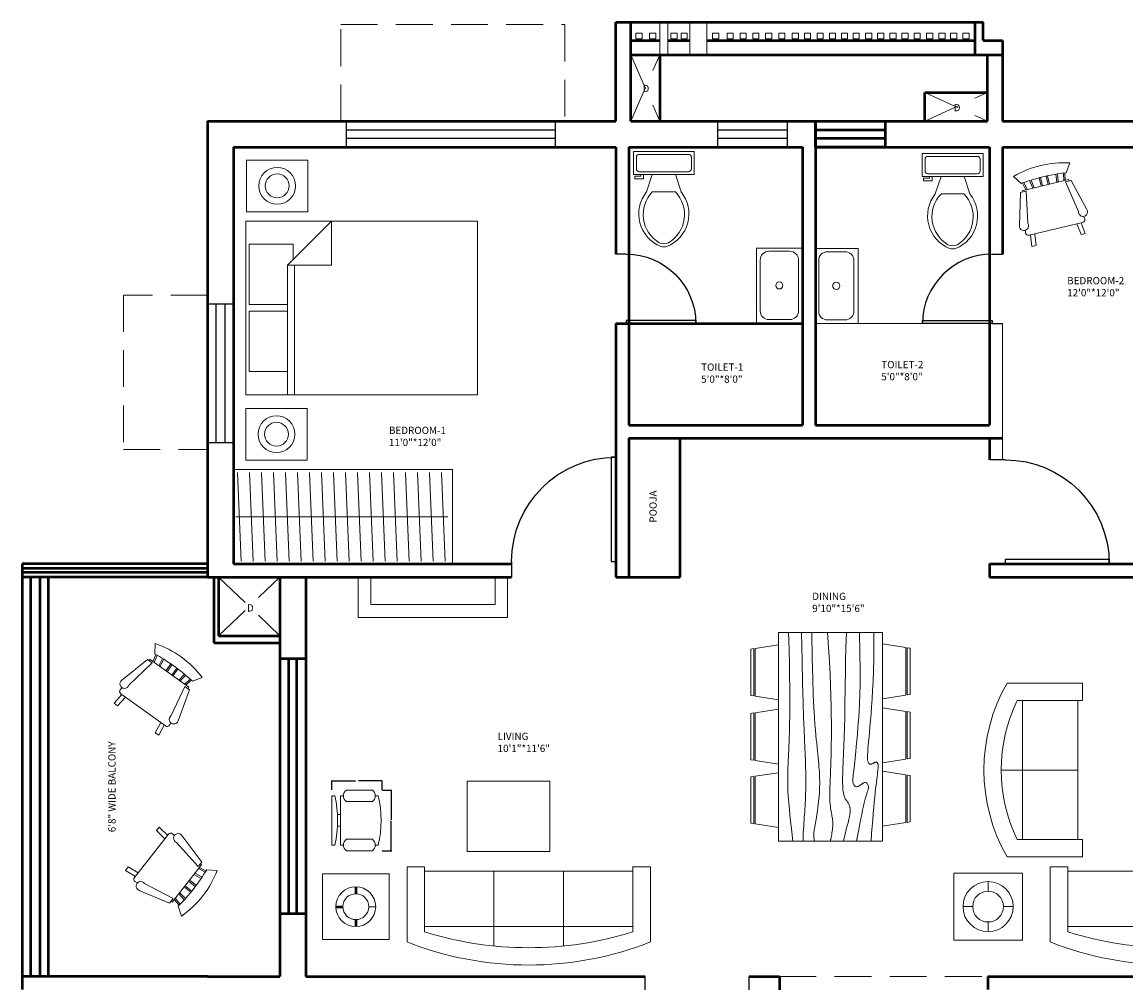
# Model space of a CAD drawing. Units: inches. Extents: x 4795 to 6024, y 2716 to 5025.
# Tile 13 of 19: x 4795 to 5177, y 4676 to 5008. Entities that reach past the tile are written whole.
import ezdxf

# ---------------------------------------------------------------- set-up
doc = ezdxf.new("R2010")
doc.units = ezdxf.units.IN
doc.linetypes.add('DASHED', pattern=[19.05, 12.7, -6.35])
for name, color, linetype, lineweight in [('A-ANNO-DIMS', 2, 'Continuous', 18), ('A-ANNO-TEXT', 7, 'Continuous', 18), ('A-AREA-IDEN', 3, 'Continuous', 18), ('A-DOOR', 4, 'Continuous', 25), ('A-FLOR-FIXT', 9, 'Continuous', 18), ('A-FURN', 8, 'Continuous', 18), ('A-GLAZ', 4, 'Continuous', 25), ('A-WALL', 7, 'Continuous', 50), ('A-WALL-OVHD', 8, 'DASHED', 18)]:
    doc.layers.add(name, color=color, linetype=linetype, lineweight=lineweight)
doc.styles.get("Standard").update_dxf_attribs({"font": 'arial.ttf'})
doc.dimstyles.get("Standard").update_dxf_attribs({"dimtxt": 0.18, "dimasz": 0.18, "dimexe": 0.18, "dimexo": 0.0625, "dimgap": 0.09, "dimtad": 0, "dimtih": 1, "dimtoh": 1, "dimdec": 4, "dimzin": 0, "dimdsep": 46, "dimtxsty": 'Standard', "dimcen": 0.09, "dimadec": 0, "dimazin": 0, "dimtfac": 1, "dimtdec": 4, "dimtofl": 0, "dimtmove": 0, "dimatfit": 3, "dimfxl": 1, "dimtolj": 1, "dimtzin": 0, "dimarcsym": 0})

# ---------------------------------------------------------------- blocks, each defined once
blk = doc.blocks.new('*U2')
for p, q in [((0, 0), (0, -6)), ((40, 0), (40, -6))]:
    blk.add_line(p, q)
blk.add_lwpolyline([(0, 0), (0, 40), (1.75, 40), (1.75, 0)], close=True)
blk.add_arc((0, 0), 40, 0, 90)
blk = doc.blocks.new('Bed - Queen')
for p, q in [((0, -80.00003), (0, 0)), ((0, 0), (59.99999, 0)), ((59.99999, 0), (59.99999, -80.00003)), ((7.99999, -1.2), (28.79998, -1.2)), ((7.99999, -14.4), (7.99999, -1.2)), ((28.79998, -1.2), (28.79998, -14.4)), ((31.19999, -1.2), (51.99999, -1.2)), ((31.19999, -14.4), (31.19999, -1.2)), ((51.99999, -1.2), (51.99999, -16.4)), ((0, -14.4), (44.8, -14.4)), ((59.99999, -29.6), (44.8, -14.4)), ((44.8, -14.4), (44.8, -29.6)), ((44.8, -16.8), (0, -16.8)), ((51.99999, -16.4), (46.79936, -16.4)), ((44.8, -29.6), (59.99999, -29.6)), ((59.99999, -80.00003), (0, -80.00003))]:
    blk.add_line(p, q)
blk = doc.blocks.new('Toilet - top')
for p, q in [((9.5, -6), (9.5, -2)), ((-10, -8.5), (-8, -8.5)), ((-10, -9.5), (-10, -8.5)), ((-7, -9.5), (-10, -9.5)), ((-8, -8.5), (-8, -8)), ((-7, -8), (-7, -9.5)), ((-4, -8), (-6, -14)), ((4, -8), (6, -14)), ((4, -14), (-4, -14))]:
    blk.add_line(p, q)
blk.add_lwpolyline([(10.5, -8), (10.5, 0), (-10.5, 0), (-10.5, -8)], close=True)
for points in [[(-9.5, -2), (-9.5, -6)], [(8.5, -1), (-8.5, -1)], [(-8.5, -7), (8.5, -7)]]:
    blk.add_lwpolyline(points)
for centre, radius, start, end in [((-8.62, -1.88), 0.884, 81.8699, 188.1301), ((8.62, -1.88), 0.884, 351.8699, 98.1301), ((-8.62, -6.12), 0.884, 171.8699, 278.1301), ((8.62, -6.12), 0.884, 261.8699, 8.1301), ((3.52, -21.58), 12.17, 141.4691, 247.9714), ((4.2, -21.82), 11.33, 136.3677, 238.9468), ((-3.52, -21.58), 12.17, 292.0284, 38.5307), ((-4.2, -21.82), 11.33, 301.053, 43.6321), ((0, -27.88), 4, 245.7318, 294.2682), ((0, -29), 4, 254.8605, 285.1395)]:
    blk.add_arc(centre, radius, start, end)
blk = doc.blocks.new('Sofa - Roundback 7 ft.')
for p, q in [((-12.00002, -32.4421), (-12.00003, -6.5971)), ((11.99997, -32.4421), (11.99998, -6.5971)), ((-36.000027, -34), (-36.000027, -11.4696)), ((-35.999844, -13.3819), (35.9998, -13.3819)), ((35.99998, -34), (35.99998, -11.4696)), ((-36.000027, -32.4421), (35.99998, -32.4421))]:
    blk.add_line(p, q)
for points in [[(-36.000027, -34), (-42.000027, -34), (-42.000027, -8)], [(41.99998, -8), (41.99998, -34), (35.99998, -34)]]:
    blk.add_lwpolyline(points)
for centre, radius, start, end in [((0, -114.25), 114.25, 68.43141, 111.5686), ((-0.00001, -127.1968), 121.1968, 72.72033, 107.2797)]:
    blk.add_arc(centre, radius, start, end)
blk = doc.blocks.new('Chair - Desk')
for p, q in [((-8.5, 0), (-8.5, -1)), ((-8.5, 0), (8.5, 0)), ((8.5, 0), (8.5, -1)), ((-8.5, -3), (-8.5, -4)), ((-8.5, -3), (8.5, -3)), ((-2, -3), (-2, -1.9355)), ((2, -1.9576), (2, -3)), ((8.5, -3), (8.5, -4)), ((-10.5, -5), (-10.5, -14)), ((-6.5, -14), (-6.5, -5)), ((6.5, -5), (6.5, -14)), ((10.5, -14), (10.5, -5)), ((-8.5, -15), (-8.5, -16)), ((8.5, -15), (8.5, -16))]:
    blk.add_line(p, q)
for centre, radius, start, end in [((0, 34.625), 36.625, 256.5803, 283.4197), ((-8.5, -6.5), 2.5, 36.8699, 143.1301), ((8.5, -6.5), 2.5, 36.8699, 143.1301), ((-8.5, -12.5), 2.5, 216.8699, 323.1301), ((8.5, -12.5), 2.5, 216.8699, 323.1301), ((0, 19.625), 36.625, 256.5803, 283.4197)]:
    blk.add_arc(centre, radius, start, end)
blk = doc.blocks.new('Sofa - Roundback Loveseat 5 ft.')
for p, q in [((0, -32.44198), (0, -5.99998)), ((-24, -33.99998), (-24, -11.46958)), ((-23.9998, -13.38178), (23.99986, -13.38178)), ((24.00004, -33.99998), (24.00004, -11.46958)), ((-24, -32.44198), (24.00004, -32.44198))]:
    blk.add_line(p, q)
for points in [[(-24, -33.99998), (-30, -33.99998), (-30, -7.99998)], [(30.00004, -7.99998), (30.00004, -33.99998), (24.00004, -33.99998)]]:
    blk.add_lwpolyline(points)
for centre, radius, start, end in [((0, -60.24998), 60.24998, 60.13715, 119.8628), ((0, -61.38438), 55.38444, 64.32083, 115.6792)]:
    blk.add_arc(centre, radius, start, end)
blk = doc.blocks.new('Chair - Rocking')
for p, q in [((-8, -4.5), (-10, -1.5)), ((8, -4.5), (10, -1.5)), ((-9, -7.5), (-12, -18.49999)), ((-7, -7.5), (-9, -7.5)), ((-9, -18.49999), (-7, -7.5)), ((-8.23428, -6.99939), (-8.3093, -7.47958)), ((-8.23041, -7), (8.23915, -7)), ((-7.5, -4.5), (-7, -7)), ((-6.5, -7), (-7.02225, -4.43)), ((-4.5, -7), (-4.96674, -4.19951)), ((-4, -7), (-4.40532, -4.16272)), ((-1.5, -4.05012), (-1.5, -7)), ((-1, -7), (-1, -4.05012)), ((1, -7), (1, -4.04655)), ((1.5, -4.05012), (1.5, -7)), ((4, -7), (4.40187, -4.18694)), ((4.5, -7), (4.96761, -4.19437)), ((6.5, -7), (7, -4.4057)), ((7.5, -4.5), (7, -7)), ((7, -7.5), (9, -7.5)), ((9, -18.49999), (7, -7.5)), ((8.31071, -7.48854), (8.23449, -7.00073)), ((9, -7.5), (12, -18.49999)), ((-10.36644, -20.64523), (-10.5, -21.49999)), ((-9, -22.49999), (-9.5, -26.49999)), ((0, -22.49999), (-9.5, -22.49999)), ((-8, -26.49999), (-7.5, -22.49999)), ((0, -22.49999), (9.5, -22.49999)), ((8, -26.49999), (7.5, -22.49999)), ((9, -22.49999), (9.5, -26.49999)), ((10.5, -21.49999), (10.3575, -20.58798)), ((-9.5, -26.49999), (-8, -26.49999)), ((9.5, -26.49999), (8, -26.49999))]:
    blk.add_line(p, q)
for centre, radius, start, end in [((0, -34.08333), 34.08333, 72.93847, 107.0615), ((0, -68.25004), 64.25, 93.92211, 97.15267), ((0, -68.25004), 64.25, 82.84733, 93.92211), ((-10.5, -18.99999), 1.58114, 161.5651, 18.43495), ((10.5, -18.99999), 1.58114, 161.5651, 18.43495), ((-9.5, -21.49999), 1, 180, 270), ((9.5, -21.49999), 1, 270, 0)]:
    blk.add_arc(centre, radius, start, end)
blk = doc.blocks.new('WIN-48')
for p, q in [((0, 0), (0, 48)), ((0, 48), (9, 48)), ((3, 0), (3, 48)), ((6, 48), (6, 0)), ((9, 48), (9, 0)), ((9, 0), (0, 0))]:
    blk.add_line(p, q)
blk = doc.blocks.new('WIN-72')
for p, q in [((0, 0), (0, 9)), ((0, 9), (72, 9)), ((72, 9), (72, 0)), ((0, 6), (72, 6)), ((72, 3), (0, 3)), ((72, 0), (0, 0))]:
    blk.add_line(p, q)
blk = doc.blocks.new('WIN-24')
for p, q in [((0, 0), (0, 9)), ((0, 9), (24, 9)), ((24, 9), (24, 0)), ((0, 6), (24, 6)), ((24, 3), (0, 3)), ((24, 0), (0, 0))]:
    blk.add_line(p, q)
blk = doc.blocks.new('CHAIR-DINING')
for p, q in [((8, 17.72), (0, 18.97)), ((8, 17.71), (8, 1.25)), ((9.5, 17.48), (8.5, 17.64)), ((8.5, 1.33), (8.5, 17.64)), ((9.5, 17.48), (9.5, 1.48)), ((0, 0), (8, 1.25)), ((8.5, 1.33), (9.5, 1.48))]:
    blk.add_line(p, q)
blk = doc.blocks.new('LAMP-SIDE')
for p, q in [((11.88, 20.25), (11.88, 16.92)), ((3.23, 11.6), (6.56, 11.6)), ((17.2, 11.6), (20.54, 11.6)), ((11.88, 6.28), (11.88, 2.94))]:
    blk.add_line(p, q)
blk.add_lwpolyline([(23.76, 23.19), (0, 23.19), (0, 0), (23.76, 0)], close=True)
for radius in [8.66, 5.32]:
    blk.add_circle((11.88, 11.6), radius)
blk = doc.blocks.new('*D19')
at = {"layer": 'A-ANNO-DIMS', "color": 0, "lineweight": -2, "transparency": 16777216}
for p, q in [((4919.79, 4742.88), (4923.06, 4742.88)), ((4922.88, 4742.7), (4922.88, 4732.56)), ((4922.88, 4722.06), (4922.88, 4732.2)), ((4919.79, 4721.88), (4923.06, 4721.88))]:
    blk.add_line(p, q, dxfattribs=at)
at = {"layer": 'A-ANNO-DIMS', "color": 0, "lineweight": 100, "transparency": 16777216}
for points in [[(4922.85, 4742.7), (4922.91, 4742.7), (4922.88, 4742.88)], [(4922.85, 4722.06), (4922.91, 4722.06), (4922.88, 4721.88)]]:
    blk.add_solid(points, dxfattribs=at)
at = {"layer": 'DEFPOINTS', "color": 0, "lineweight": 100, "transparency": 16777216}
for p in [(4919.73, 4742.88), (4922.88, 4742.88), (4919.73, 4721.88)]:
    blk.add_point(p, dxfattribs=at)
at = {"layer": 'A-ANNO-DIMS', "color": 0, "transparency": 16777216, "insert": (4922.88, 4732.38), "char_height": 0.18, "attachment_point": 5}
blk.add_mtext('\\A1;DESK CHAIR 21 TYP.', dxfattribs=at)
blk = doc.blocks.new('*D20')
at = {"layer": 'A-ANNO-DIMS', "color": 0, "lineweight": -2, "transparency": 16777216}
for p, q in [((4902.4, 4742.94), (4902.4, 4746.21)), ((4902.58, 4746.03), (4910.54, 4746.03)), ((4919.55, 4746.03), (4911.58, 4746.03)), ((4919.73, 4742.94), (4919.73, 4746.21))]:
    blk.add_line(p, q, dxfattribs=at)
at = {"layer": 'A-ANNO-DIMS', "color": 0, "lineweight": 100, "transparency": 16777216}
for points in [[(4902.58, 4746.06), (4902.58, 4746), (4902.4, 4746.03)], [(4919.55, 4746.06), (4919.55, 4746), (4919.73, 4746.03)]]:
    blk.add_solid(points, dxfattribs=at)
at = {"layer": 'DEFPOINTS', "color": 0, "lineweight": 100, "transparency": 16777216}
for p in [(4902.4, 4746.03), (4902.4, 4742.88), (4919.73, 4742.88)]:
    blk.add_point(p, dxfattribs=at)
at = {"layer": 'A-ANNO-DIMS', "color": 0, "transparency": 16777216, "insert": (4911.06, 4746.03), "char_height": 0.18, "attachment_point": 5}
blk.add_mtext('\\A1;17 TYP.', dxfattribs=at)

msp = doc.modelspace()

# ---------------------------------------------------------------- linework, layer by layer
at = {"layer": 'A-FLOR-FIXT'}
for points in [[(5064.97, 4904.04), (5049.09, 4904.04), (5049.09, 4930.14), (5064.97, 4930.14)], [(5069.47, 4904.04), (5084.11, 4904.04), (5084.11, 4929.94), (5069.47, 4929.94)]]:
    msp.add_lwpolyline(points, close=True, dxfattribs=at)
for points in [[(5053.31, 4929.01), (5060.55, 4929.01, -0.414214), (5063.55, 4926.01), (5063.55, 4908.43, -0.414214), (5060.55, 4905.43), (5053.31, 4905.43, -0.414214), (5050.31, 4908.43), (5050.31, 4926.01, -0.414214)], [(5073.51, 4928.86), (5079.66, 4928.86, -0.414214), (5082.66, 4925.86), (5082.66, 4908.32, -0.414214), (5079.66, 4905.32), (5073.51, 4905.32, -0.414214), (5070.51, 4908.32), (5070.51, 4925.86, -0.414214)]]:
    msp.add_lwpolyline(points, format="xyb", close=True, dxfattribs=at)
for centre, radius in [((5056.93, 4917.22), 1.22), ((5076.59, 4917.09), 1.24)]:
    msp.add_circle(centre, radius, dxfattribs=at)
at = {"layer": 'A-FURN'}
for p, q in [((5069.47, 4904.04), (5133.97, 4904.04)), ((5133.97, 4904.04), (5133.97, 4856.98)), ((4868.47, 4853.67), (4944.05, 4853.67)), ((4869.87, 4852.58), (4871.08, 4821.91)), ((4874.01, 4852.58), (4875.23, 4821.91)), ((4878.15, 4852.58), (4879.37, 4821.91)), ((4882.3, 4852.58), (4883.51, 4821.91)), ((4886.44, 4852.58), (4887.66, 4821.91)), ((4890.58, 4852.58), (4891.8, 4821.91)), ((4894.73, 4852.58), (4895.94, 4821.91)), ((4898.87, 4852.58), (4900.09, 4821.91)), ((4903.02, 4852.58), (4904.23, 4821.91)), ((4907.16, 4852.58), (4908.38, 4821.91)), ((4911.3, 4852.58), (4912.52, 4821.91)), ((4915.45, 4852.58), (4916.66, 4821.91)), ((4919.59, 4852.58), (4920.81, 4821.91)), ((4923.73, 4852.58), (4924.95, 4821.91)), ((4927.88, 4852.58), (4929.09, 4821.91)), ((4932.02, 4852.58), (4933.24, 4821.91)), ((4936.17, 4852.58), (4937.38, 4821.91)), ((4940.31, 4852.58), (4941.53, 4821.91)), ((4944.05, 4853.67), (4944.05, 4820.98)), ((4869.24, 4837.25), (4942.48, 4837.25)), ((4911.47, 4816.48), (4911.47, 4802.48)), ((4915.82, 4816.48), (4915.82, 4806.99)), ((4958.77, 4806.99), (4958.77, 4816.48)), ((4963.08, 4802.48), (4963.08, 4816.48)), ((4915.82, 4806.99), (4958.77, 4806.99)), ((4911.47, 4802.48), (4963.08, 4802.48)), ((5056.6, 4797.26), (5056.6, 4725.26)), ((5092.6, 4797.26), (5056.6, 4797.26)), ((5092.6, 4725.26), (5092.6, 4797.26)), ((5056.6, 4725.26), (5092.6, 4725.26)), ((4915.14, 4702.58), (4917.55, 4702.58))]:
    msp.add_line(p, q, dxfattribs=at)
for points in [[(5015.65, 5008.22), (5018.42, 5008.22), (5018.42, 4996.94), (5015.65, 4996.94)], [(5026.04, 5008.22), (5031.9, 5008.22), (5031.9, 4996.94), (5026.04, 4996.94)], [(5007.39, 5004.38), (5009.52, 5004.38), (5009.52, 5002.46), (5007.39, 5002.46)], [(5012.14, 5004.38), (5014.27, 5004.38), (5014.27, 5002.46), (5012.14, 5002.46)], [(5019.47, 5004.38), (5021.6, 5004.38), (5021.6, 5002.46), (5019.47, 5002.46)], [(5022.98, 5004.38), (5025.1, 5004.38), (5025.1, 5002.46), (5022.98, 5002.46)], [(5033.88, 5004.38), (5036, 5004.38), (5036, 5002.46), (5033.88, 5002.46)], [(5038.86, 5004.38), (5040.99, 5004.38), (5040.99, 5002.46), (5038.86, 5002.46)], [(5043.35, 5004.38), (5045.47, 5004.38), (5045.47, 5002.46), (5043.35, 5002.46)], [(5047.73, 5004.38), (5049.86, 5004.38), (5049.86, 5002.46), (5047.73, 5002.46)], [(5052.19, 5004.38), (5054.32, 5004.38), (5054.32, 5002.46), (5052.19, 5002.46)], [(5056.71, 5004.38), (5058.83, 5004.38), (5058.83, 5002.46), (5056.71, 5002.46)], [(5061.36, 5004.38), (5063.49, 5004.38), (5063.49, 5002.46), (5061.36, 5002.46)], [(5065.58, 5004.38), (5067.71, 5004.38), (5067.71, 5002.46), (5065.58, 5002.46)], [(5069.98, 5004.38), (5072.1, 5004.38), (5072.1, 5002.46), (5069.98, 5002.46)], [(5074.23, 5004.38), (5076.36, 5004.38), (5076.36, 5002.46), (5074.23, 5002.46)], [(5078.38, 5004.38), (5080.51, 5004.38), (5080.51, 5002.46), (5078.38, 5002.46)], [(5082.37, 5004.38), (5084.5, 5004.38), (5084.5, 5002.46), (5082.37, 5002.46)], [(5086.69, 5004.38), (5088.82, 5004.38), (5088.82, 5002.46), (5086.69, 5002.46)], [(5090.88, 5004.38), (5093.01, 5004.38), (5093.01, 5002.46), (5090.88, 5002.46)], [(5095.1, 5004.38), (5097.23, 5004.38), (5097.23, 5002.46), (5095.1, 5002.46)], [(5099.26, 5004.38), (5101.38, 5004.38), (5101.38, 5002.46), (5099.26, 5002.46)], [(5103.48, 5004.38), (5105.61, 5004.38), (5105.61, 5002.46), (5103.48, 5002.46)], [(5107.77, 5004.38), (5109.9, 5004.38), (5109.9, 5002.46), (5107.77, 5002.46)], [(5112.06, 5004.38), (5114.18, 5004.38), (5114.18, 5002.46), (5112.06, 5002.46)], [(5116.08, 5004.38), (5118.2, 5004.38), (5118.2, 5002.46), (5116.08, 5002.46)], [(5120.33, 5004.38), (5122.46, 5004.38), (5122.46, 5002.46), (5120.33, 5002.46)], [(4872.88, 4960.54), (4894.15, 4960.54), (4894.15, 4942.71), (4872.88, 4942.71)], [(4872.65, 4874.74), (4893.91, 4874.74), (4893.91, 4856.91), (4872.65, 4856.91)], [(4949.08, 4745.98), (4977.63, 4745.98), (4977.63, 4721.64), (4949.08, 4721.64)], [(4899.19, 4713.94), (4922.15, 4713.94), (4922.15, 4691.23), (4899.19, 4691.23)]]:
    msp.add_lwpolyline(points, close=True, dxfattribs=at)
for points in [[(5060.1, 4797.26), (5060.27, 4791.35), (5060.39, 4786.3), (5060.48, 4781.99), (5060.53, 4778.34), (5060.56, 4775.23), (5060.56, 4772.57), (5060.55, 4770.24), (5060.52, 4768.14), (5060.49, 4766.19), (5060.44, 4764.35), (5060.4, 4762.63), (5060.34, 4761.02), (5060.29, 4759.5), (5060.23, 4758.07), (5060.17, 4756.71), (5060.1, 4755.43), (5060.04, 4754.21), (5059.98, 4753.03), (5059.93, 4751.87), (5059.88, 4750.72), (5059.84, 4749.54), (5059.82, 4748.33), (5059.81, 4747.07), (5059.81, 4745.72), (5059.84, 4744.27), (5059.9, 4742.65), (5060, 4740.78), (5060.16, 4738.6), (5060.39, 4736.03), (5060.7, 4733), (5061.1, 4729.44), (5061.6, 4725.26)], [(5064.6, 4797.26), (5064.79, 4787.67), (5064.98, 4779.73), (5065.15, 4773.25), (5065.32, 4768), (5065.48, 4763.79), (5065.62, 4760.38), (5065.75, 4757.59), (5065.85, 4755.18), (5065.94, 4752.99), (5066, 4750.96), (5066.04, 4749.09), (5066.06, 4747.37), (5066.07, 4745.78), (5066.06, 4744.3), (5066.05, 4742.94), (5066.02, 4741.68), (5065.99, 4740.5), (5065.94, 4739.39), (5065.89, 4738.34), (5065.84, 4737.34), (5065.78, 4736.35), (5065.71, 4735.39), (5065.64, 4734.42), (5065.56, 4733.43), (5065.48, 4732.42), (5065.4, 4731.38), (5065.33, 4730.33), (5065.26, 4729.28), (5065.19, 4728.24), (5065.15, 4727.22), (5065.12, 4726.22), (5065.1, 4725.26)], [(5068.1, 4797.26), (5068.29, 4788.45), (5068.48, 4781.35), (5068.66, 4775.73), (5068.84, 4771.37), (5069.02, 4768.04), (5069.19, 4765.5), (5069.36, 4763.53), (5069.52, 4761.89), (5069.67, 4760.39), (5069.82, 4758.99), (5069.95, 4757.68), (5070.08, 4756.43), (5070.2, 4755.26), (5070.32, 4754.14), (5070.42, 4753.06), (5070.52, 4752.01), (5070.61, 4750.99), (5070.69, 4749.99), (5070.76, 4749), (5070.81, 4748.01), (5070.85, 4747.03), (5070.87, 4746.04), (5070.87, 4745.03), (5070.85, 4744.01), (5070.81, 4742.97), (5070.75, 4741.92), (5070.67, 4740.86), (5070.57, 4739.82), (5070.47, 4738.79), (5070.35, 4737.79), (5070.23, 4736.83), (5070.1, 4735.93), (5069.98, 4735.08), (5069.85, 4734.29), (5069.73, 4733.55), (5069.61, 4732.84), (5069.49, 4732.16), (5069.37, 4731.51), (5069.26, 4730.86), (5069.15, 4730.22), (5069.04, 4729.58), (5068.95, 4728.94), (5068.87, 4728.3), (5068.83, 4727.66), (5068.82, 4727.04), (5068.86, 4726.43), (5068.95, 4725.84), (5069.1, 4725.26)], [(5073.6, 4797.26), (5073.94, 4792.05), (5074.22, 4787.28), (5074.44, 4782.91), (5074.61, 4778.92), (5074.73, 4775.26), (5074.82, 4771.92), (5074.87, 4768.84), (5074.9, 4766.01), (5074.9, 4763.4), (5074.89, 4760.98), (5074.87, 4758.73), (5074.83, 4756.65), (5074.78, 4754.71), (5074.73, 4752.9), (5074.67, 4751.2), (5074.6, 4749.6), (5074.54, 4748.07), (5074.48, 4746.63), (5074.43, 4745.26), (5074.39, 4743.98), (5074.35, 4742.78), (5074.33, 4741.66), (5074.33, 4740.63), (5074.35, 4739.68), (5074.4, 4738.81), (5074.46, 4738.03), (5074.54, 4737.31), (5074.62, 4736.65), (5074.72, 4736.04), (5074.82, 4735.47), (5074.92, 4734.94), (5075.02, 4734.43), (5075.11, 4733.94), (5075.19, 4733.45), (5075.26, 4732.97), (5075.31, 4732.49), (5075.35, 4732), (5075.37, 4731.5), (5075.37, 4730.98), (5075.35, 4730.43), (5075.31, 4729.85), (5075.25, 4729.26), (5075.18, 4728.67), (5075.09, 4728.1), (5075.01, 4727.56), (5074.92, 4727.07), (5074.84, 4726.65), (5074.77, 4726.3), (5074.72, 4726.05), (5074.67, 4725.88), (5074.64, 4725.76), (5074.62, 4725.67), (5074.61, 4725.6), (5074.61, 4725.53), (5074.6, 4725.42), (5074.6, 4725.26)], [(5080.1, 4797.26), (5079.94, 4791.98), (5079.81, 4787.33), (5079.72, 4783.26), (5079.66, 4779.69), (5079.61, 4776.56), (5079.58, 4773.81), (5079.55, 4771.37), (5079.52, 4769.18), (5079.49, 4767.17), (5079.44, 4765.32), (5079.4, 4763.61), (5079.34, 4762), (5079.29, 4760.49), (5079.23, 4759.04), (5079.17, 4757.64), (5079.1, 4756.26), (5079.04, 4754.89), (5078.98, 4753.53), (5078.93, 4752.19), (5078.87, 4750.89), (5078.83, 4749.63), (5078.8, 4748.43), (5078.78, 4747.31), (5078.77, 4746.26), (5078.78, 4745.31), (5078.8, 4744.44), (5078.84, 4743.66), (5078.9, 4742.96), (5078.97, 4742.33), (5079.05, 4741.77), (5079.15, 4741.28), (5079.27, 4740.85), (5079.4, 4740.47), (5079.55, 4740.13), (5079.7, 4739.84), (5079.86, 4739.58), (5080.03, 4739.34), (5080.2, 4739.11), (5080.36, 4738.9), (5080.52, 4738.68), (5080.67, 4738.46), (5080.81, 4738.22), (5080.95, 4737.98), (5081.06, 4737.71), (5081.16, 4737.43), (5081.25, 4737.12), (5081.31, 4736.79), (5081.35, 4736.43), (5081.37, 4736.04), (5081.37, 4735.62), (5081.35, 4735.18), (5081.3, 4734.71), (5081.24, 4734.23), (5081.15, 4733.72), (5081.05, 4733.21), (5080.94, 4732.68), (5080.8, 4732.14), (5080.65, 4731.56), (5080.47, 4730.9), (5080.27, 4730.13), (5080.04, 4729.21), (5079.77, 4728.12), (5079.46, 4726.82), (5079.1, 4725.26)], [(5084.6, 4797.26), (5084.75, 4790.24), (5084.81, 4784.44), (5084.8, 4779.69), (5084.74, 4775.83), (5084.63, 4772.7), (5084.5, 4770.14), (5084.35, 4767.98), (5084.19, 4766.05), (5084.03, 4764.23), (5083.89, 4762.49), (5083.75, 4760.82), (5083.61, 4759.24), (5083.48, 4757.74), (5083.36, 4756.32), (5083.23, 4755), (5083.1, 4753.76), (5082.98, 4752.62), (5082.86, 4751.57), (5082.74, 4750.61), (5082.64, 4749.73), (5082.54, 4748.94), (5082.46, 4748.22), (5082.4, 4747.58), (5082.35, 4747.01), (5082.33, 4746.52), (5082.34, 4746.08), (5082.36, 4745.71), (5082.41, 4745.39), (5082.47, 4745.11), (5082.55, 4744.88), (5082.65, 4744.68), (5082.77, 4744.51), (5082.9, 4744.37), (5083.05, 4744.25), (5083.21, 4744.15), (5083.37, 4744.09), (5083.55, 4744.04), (5083.73, 4744.03), (5083.92, 4744.05), (5084.1, 4744.1), (5084.29, 4744.17), (5084.48, 4744.28), (5084.67, 4744.4), (5084.85, 4744.53), (5085.04, 4744.68), (5085.23, 4744.82), (5085.42, 4744.96), (5085.6, 4745.1), (5085.79, 4745.21), (5085.98, 4745.31), (5086.16, 4745.39), (5086.34, 4745.44), (5086.52, 4745.46), (5086.69, 4745.46), (5086.86, 4745.42), (5087.02, 4745.35), (5087.17, 4745.23), (5087.31, 4745.08), (5087.44, 4744.9), (5087.54, 4744.69), (5087.62, 4744.45), (5087.68, 4744.19), (5087.7, 4743.9), (5087.69, 4743.6), (5087.64, 4743.27), (5087.55, 4742.92), (5087.43, 4742.52), (5087.29, 4742.07), (5087.11, 4741.54), (5086.92, 4740.93), (5086.71, 4740.22), (5086.48, 4739.39), (5086.24, 4738.43), (5085.98, 4737.3), (5085.69, 4735.98), (5085.37, 4734.43), (5085.01, 4732.62), (5084.6, 4730.51), (5084.13, 4728.07), (5083.6, 4725.26)], [(5089.6, 4797.26), (5089.58, 4792.44), (5089.52, 4788.07), (5089.42, 4784.12), (5089.29, 4780.54), (5089.14, 4777.3), (5088.97, 4774.36), (5088.79, 4771.68), (5088.6, 4769.22), (5088.42, 4766.95), (5088.23, 4764.87), (5088.06, 4762.96), (5087.9, 4761.23), (5087.75, 4759.67), (5087.62, 4758.28), (5087.51, 4757.06), (5087.44, 4756.01), (5087.39, 4755.12), (5087.37, 4754.38), (5087.38, 4753.77), (5087.42, 4753.28), (5087.47, 4752.89), (5087.55, 4752.59), (5087.65, 4752.36), (5087.77, 4752.18), (5087.9, 4752.04), (5088.05, 4751.94), (5088.2, 4751.87), (5088.36, 4751.84), (5088.53, 4751.83), (5088.7, 4751.84), (5088.86, 4751.88), (5089.02, 4751.93), (5089.17, 4752), (5089.32, 4752.08), (5089.46, 4752.17), (5089.59, 4752.25), (5089.72, 4752.34), (5089.85, 4752.41), (5089.98, 4752.47), (5090.1, 4752.51), (5090.23, 4752.53), (5090.35, 4752.53), (5090.47, 4752.5), (5090.58, 4752.45), (5090.69, 4752.38), (5090.78, 4752.28), (5090.87, 4752.16), (5090.94, 4752.01), (5090.99, 4751.84), (5091.03, 4751.65), (5091.05, 4751.41), (5091.06, 4751.14), (5091.05, 4750.82), (5091.03, 4750.44), (5090.99, 4750.01), (5090.94, 4749.51), (5090.87, 4748.94), (5090.78, 4748.29), (5090.68, 4747.55), (5090.57, 4746.7), (5090.45, 4745.72), (5090.32, 4744.62), (5090.17, 4743.37), (5090.02, 4741.97), (5089.86, 4740.4), (5089.69, 4738.68), (5089.52, 4736.79), (5089.34, 4734.76), (5089.16, 4732.58), (5088.98, 4730.27), (5088.79, 4727.83), (5088.6, 4725.26)]]:
    msp.add_lwpolyline(points, dxfattribs=at)
for centre, radius in [((4883.52, 4951.63), 6.37), ((4883.52, 4951.63), 4.11), ((4883.28, 4865.82), 6.37), ((4883.28, 4865.82), 4.11), ((4910.67, 4702.58), 6.88), ((4910.67, 4702.58), 4.47)]:
    msp.add_circle(centre, radius, dxfattribs=at)
at = {"layer": 'A-WALL'}
for p, q in [((5000.47, 4973.98), (5000.47, 5008.22)), ((5000.47, 5008.22), (5127.34, 5008.22)), ((5005.65, 4973.98), (5005.65, 5008.22)), ((5124.46, 5008.22), (5124.46, 4996.94)), ((5127.34, 5001.88), (5127.34, 5008.22)), ((5005.65, 5001.88), (5015.65, 5001.88)), ((5018.42, 5001.88), (5026.04, 5001.88)), ((5031.9, 5001.88), (5124.46, 5001.88)), ((5127.34, 5001.88), (5133.97, 5001.88)), ((5133.97, 5001.88), (5133.97, 4973.98)), ((5005.65, 4996.94), (5133.97, 4996.94)), ((5015.65, 4996.94), (5015.65, 4973.98)), ((5128.82, 4973.98), (5128.82, 4996.94)), ((5107.16, 4973.98), (5107.16, 4983.85)), ((5107.16, 4983.85), (5128.82, 4983.85)), ((4859.47, 4973.98), (4859.47, 4816.48)), ((4859.47, 4973.98), (5000.47, 4973.98)), ((5005.65, 4973.98), (5128.82, 4973.98)), ((5069.47, 4973.98), (5069.47, 4868.98)), ((5069.47, 4973.98), (5093.47, 4973.98)), ((5069.47, 4964.98), (5069.47, 4973.98)), ((5069.47, 4970.98), (5093.47, 4970.98)), ((5093.47, 4973.98), (5093.47, 4964.98)), ((5133.97, 4973.98), (5286.97, 4973.98)), ((5093.47, 4967.98), (5069.47, 4967.98)), ((4868.47, 4964.98), (5000.47, 4964.98)), ((4868.47, 4964.98), (4868.47, 4820.98)), ((5000.47, 4964.98), (5000.47, 4928.04)), ((5004.97, 4964.98), (5004.97, 4868.98)), ((5004.97, 4964.98), (5064.97, 4964.98)), ((5064.97, 4964.98), (5064.97, 4868.98)), ((5093.47, 4964.98), (5069.47, 4964.98)), ((5069.47, 4964.98), (5129.47, 4964.98)), ((5129.47, 4964.98), (5129.47, 4868.98)), ((5133.97, 4964.98), (5133.97, 4928.04)), ((5133.97, 4964.98), (5277.97, 4964.98)), ((5000.47, 4904.04), (5064.97, 4904.04)), ((5000.47, 4904.04), (5000.47, 4816.48)), ((5004.97, 4868.98), (5064.97, 4868.98)), ((5069.47, 4868.98), (5129.47, 4868.98)), ((5004.97, 4864.48), (5133.97, 4864.48)), ((5004.97, 4864.48), (5004.97, 4816.48)), ((5022.69, 4816.48), (5022.69, 4864.48)), ((5129.47, 4864.48), (5129.47, 4856.98)), ((4795.42, 4820.98), (4795.42, 4673.98)), ((4859.47, 4820.98), (4795.42, 4820.98)), ((4795.42, 4819.56), (4859.47, 4819.56)), ((4868.47, 4820.98), (4964.47, 4820.98)), ((5129.47, 4820.98), (5277.97, 4820.98)), ((5129.47, 4820.98), (5129.47, 4816.48)), ((4795.42, 4818.19), (4859.47, 4818.19)), ((4859.47, 4816.48), (4795.42, 4816.48)), ((4798.38, 4816.48), (4798.38, 4678.48)), ((4801.51, 4816.48), (4801.51, 4678.48)), ((4804.42, 4816.48), (4804.42, 4678.48)), ((4859.47, 4816.48), (4964.47, 4816.48)), ((4861.65, 4816.48), (4861.65, 4793.7)), ((4863.28, 4816.48), (4863.28, 4796.16)), ((4884.42, 4816.48), (4884.42, 4678.48)), ((4893.42, 4816.48), (4893.42, 4678.48)), ((5000.47, 4816.48), (5004.97, 4816.48)), ((5004.97, 4816.48), (5022.69, 4816.48)), ((5129.47, 4816.48), (5277.97, 4816.48)), ((4863.28, 4796.16), (4884.42, 4796.16)), ((4861.65, 4793.7), (4884.42, 4793.7)), ((4884.42, 4788.28), (4893.42, 4788.28)), ((4887.38, 4788.28), (4887.38, 4700.21)), ((4890.17, 4788.28), (4890.17, 4700.21)), ((4910.67, 4709.46), (4910.67, 4707.05)), ((4884.42, 4700.21), (4893.42, 4700.21)), ((4903.8, 4702.58), (4906.21, 4702.58)), ((4910.67, 4698.12), (4910.67, 4695.71)), ((4804.42, 4678.48), (4795.42, 4678.48)), ((4859.47, 4678.48), (4804.42, 4678.48)), ((4859.47, 4678.48), (4884.42, 4678.48)), ((4893.42, 4678.48), (5010.54, 4678.48)), ((5046.54, 4678.48), (5056.97, 4678.48)), ((5056.97, 4678.48), (5056.97, 4623.48)), ((5128.97, 4678.48), (5128.97, 4673.98)), ((5128.97, 4678.48), (5277.97, 4678.48))]:
    msp.add_line(p, q, dxfattribs=at)
at = {"layer": 'A-WALL-OVHD'}
for p, q in [((4905.5, 4973.98), (4905.5, 5007.33)), ((4905.5, 5007.33), (4982.88, 5007.33)), ((4982.88, 5007.33), (4982.88, 4973.98)), ((5005.65, 4996.94), (5015.65, 4973.98)), ((5005.65, 4973.98), (5015.65, 4996.94)), ((5107.16, 4983.85), (5128.82, 4973.98)), ((5107.16, 4973.98), (5128.82, 4983.85)), ((4859.47, 4913.89), (4830.42, 4913.89)), ((4830.42, 4913.89), (4830.42, 4860.52)), ((4830.42, 4860.52), (4859.47, 4860.52)), ((4863.28, 4816.48), (4884.42, 4796.16)), ((4863.28, 4796.16), (4884.42, 4816.48)), ((5056.97, 4678.48), (5128.97, 4678.48))]:
    msp.add_line(p, q, dxfattribs=at)

# ---------------------------------------------------------------- block references
at = {"layer": 'A-DOOR'}
for p, xscale, yscale, zscale, rotation in [((5004.07, 4904.04), -0.6, 0.6, 0.6, 270), ((5130.37, 4904.04), 0.6, 0.6, 0.6, 90.00000000000003), ((5134.87, 4820.98), -0.9, 0.9, 0.9, 270), ((5046.54, 4673.08), 0.9, 0.9, 0.9, 180)]:
    msp.add_blockref('*U2', p, dxfattribs=dict(at, xscale=xscale, yscale=yscale, zscale=zscale, rotation=rotation))
at = {"layer": 'A-DOOR', "xscale": -0.9, "yscale": 0.9, "zscale": 0.9}
msp.add_blockref('*U2', (5000.47, 4821.88), dxfattribs=at)
at = {"layer": 'A-FLOR-FIXT'}
for p in [(5017.05, 4963.52), (5116.76, 4962.82)]:
    msp.add_blockref('Toilet - top', p, dxfattribs=at)
at = {"layer": 'A-FURN'}
for name, p, rotation in [('Chair - Rocking', (5147.18, 4958.68), 13.47603948756063), ('Bed - Queen', (4872.65, 4879.48), 90), ('Chair - Rocking', (4850.37, 4788.86), 324.2775344515209), ('CHAIR-DINING', (5056.61, 4793.06), 180.0056718243519), ('Sofa - Roundback Loveseat 5 ft.', (5127.57, 4749.79), 90), ('CHAIR-DINING', (5056.61, 4770.84), 180.0056718243519), ('CHAIR-DINING', (5056.61, 4748.87), 180.0056718243519), ('Chair - Desk', (4902.4, 4732.38), 90), ('Chair - Rocking', (4857.82, 4706.29), 232.0049313276433), ('Sofa - Roundback 7 ft.', (4970.39, 4682.4), 180), ('Sofa - Roundback 7 ft.', (5192.5, 4682.4), 180)]:
    msp.add_blockref(name, p, dxfattribs=dict(at, rotation=rotation))
for name, p in [('CHAIR-DINING', (5092.6, 4774.43)), ('CHAIR-DINING', (5092.6, 4752.33)), ('CHAIR-DINING', (5092.6, 4730.39)), ('LAMP-SIDE', (5117.14, 4691.01))]:
    msp.add_blockref(name, p, dxfattribs=at)
at = {"layer": 'A-GLAZ', "rotation": 180}
for name, p in [('WIN-72', (4979.49, 4973.98)), ('WIN-24', (5059.66, 4973.98))]:
    msp.add_blockref(name, p, dxfattribs=at)
at = {"layer": 'A-GLAZ'}
msp.add_blockref('WIN-48', (4859.47, 4862.88), dxfattribs=at)

# ---------------------------------------------------------------- texts
at = {"layer": 'A-ANNO-TEXT', "char_height": 2.5, "attachment_point": 1}
for width, insert in [(2.6156, (5009.68, 4986.55)), (2.1392, (5117.14, 4979.91)), (1.8347, (4873.09, 4807.05))]:
    msp.add_mtext_dynamic_manual_height_columns('D', width=width, gutter_width=12.5, heights=[0], dxfattribs=dict(at, insert=insert))
at = {"layer": 'A-AREA-IDEN', "char_height": 2.5, "attachment_point": 1}
for s, width, insert in [('BEDROOM-2\\P12\'0"*12\'0"', 46.3923, (5156.33, 4920.13)), ('TOILET-2\\P5\'0"*8\'0"', 32.5667, (5092.13, 4891.13)), ('TOILET-1\\P5\'0"*8\'0"', 43.8668, (5029.93, 4890.26)), ('BEDROOM-1\\P11\'0"*12\'0"', 49.6902, (4922.12, 4868.41)), ('DINING\\P9\'10"*15\'6"', 35.3489, (5068.29, 4811.05)), ('LIVING\\P10\'1"*11\'6"', 46.5966, (4959.64, 4762.68))]:
    msp.add_mtext_dynamic_manual_height_columns(s, width=width, gutter_width=12.5, heights=[0], dxfattribs=dict(at, insert=insert))
at = {"layer": 'A-AREA-IDEN', "char_height": 2.5, "attachment_point": 1, "rotation": 90}
for s, width, insert in [('POOJA', 12.3439, (5012.07, 4835.26)), ('6\'8" WIDE BALCONY', 55.4373, (4825.21, 4728.31))]:
    msp.add_mtext_dynamic_manual_height_columns(s, width=width, gutter_width=12.5, heights=[0], dxfattribs=dict(at, insert=insert))

# ---------------------------------------------------------------- dimensions: what is measured, and where the dimension line sits
at = {"layer": 'A-ANNO-DIMS'}
for base, p1, p2, angle, text, picture, middle in [((4902.4, 4746.03), (4919.73, 4742.88), (4902.4, 4742.88), 180, '<> TYP.', '*D20', (4911.06, 4746.03)), ((4922.88, 4742.88), (4919.73, 4721.88), (4919.73, 4742.88), 90, 'DESK CHAIR <> TYP.', '*D19', (4922.88, 4732.38))]:
    dim = msp.add_linear_dim(base=base, p1=p1, p2=p2, angle=angle, text=text, dimstyle='Standard', override={"dimdec": 0, "dimlfac": 1, "dimrnd": 0, "dimzin": 0, "dimdsep": 46, "dimlunit": 2}, dxfattribs=at)
    dim.commit()
    dim.dimension.update_dxf_attribs({"geometry": picture, "text_midpoint": middle})

doc.saveas('drawing.dxf')
